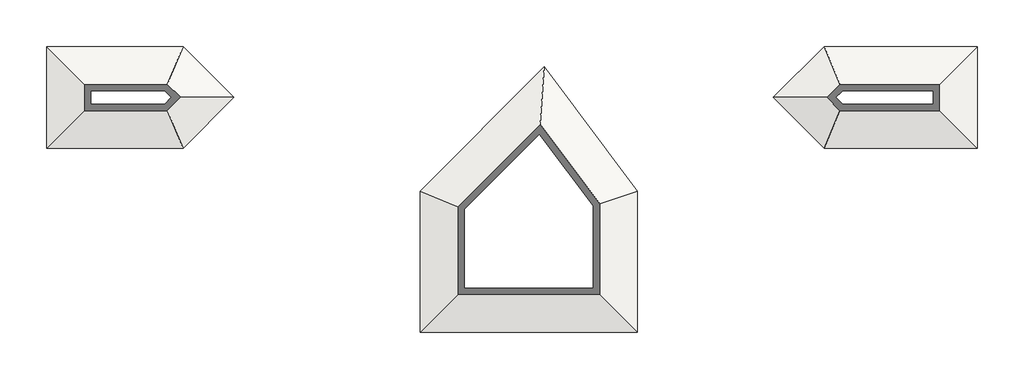
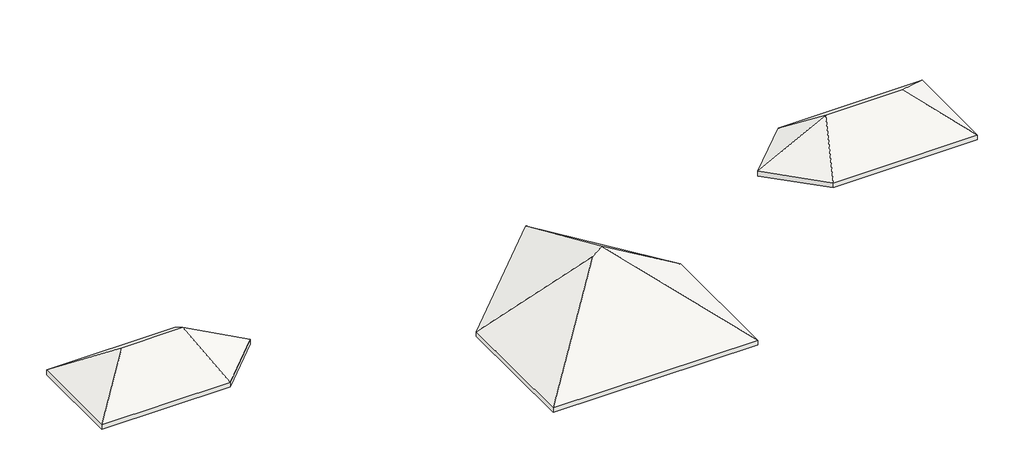
# One storey: 3 roofs.
"""IFC4 building model written with IfcOpenShell, lengths in millimetres."""

from ifc_helpers import new_model, si_unit, origin, place, context, project, spatial, faceted_brep, element, save

model = new_model("IFC4")

# Units and contexts
model_context = context("Model", 3, world=origin())
ifc_project = project(units=[si_unit("LENGTHUNIT", "METRE", prefix="MILLI")], contexts=[model_context])

# Site, building, storey
site = spatial("IfcSite", under=ifc_project)
building = spatial("IfcBuilding", under=site)
storey = spatial("IfcBuildingStorey", under=building, Elevation=7500.0)

# Roofs
placement = place(None, origin())
element("IfcRoof", 1, ObjectType="01-roof sheet", at=placement, inside=storey, context=model_context, shape_type="Brep", body=[
    faceted_brep([(-11618.9169632, -3415.5592374, 7500.0), (-6716.8860603, -3415.5592374, 7500.0), (-7472.8258116, -5240.5592374, 8868.75), (-9793.9169632, -5240.5592374, 8868.75), (-11618.9169632, -7065.5592374, 7500.0), (-6716.8860603, -7065.5592374, 7500.0), (-4891.8860603, -5240.5592374, 7500.0), (-11618.9169632, -3415.5592374, 7687.5), (-9793.9169632, -5240.5592374, 9056.25), (-7472.8258116, -5240.5592374, 9056.25), (-6716.8860603, -3415.5592374, 7687.5), (-11618.9169632, -7065.5592374, 7687.5), (-6716.8860603, -7065.5592374, 7687.5), (-4891.8860603, -5240.5592374, 7687.5)], [[[0, 1, 2, 3]], [[0, 3, 4]], [[4, 3, 2, 5]], [[6, 2, 1]], [[5, 2, 6]], [[7, 8, 9, 10]], [[7, 11, 8]], [[11, 12, 9, 8]], [[13, 10, 9]], [[12, 13, 9]], [[4, 11, 7, 0]], [[5, 12, 11, 4]], [[6, 13, 12, 5]], [[1, 10, 13, 6]], [[0, 7, 10, 1]]]),
])
element("IfcRoof", 2, ObjectType="01-roof sheet", at=placement, inside=storey, context=model_context, shape_type="Brep", body=[
    faceted_brep([(19981.0830368, -5240.5592374, 8868.75), (21806.0830368, -7065.5592374, 7500.0), (16306.0830368, -7065.5592374, 7500.0), (17062.0227881, -5240.5592374, 8868.75), (21806.0830368, -3415.5592374, 7500.0), (16306.0830368, -3415.5592374, 7500.0), (14481.0830368, -5240.5592374, 7500.0), (21806.0830368, -7065.5592374, 7687.5), (19981.0830368, -5240.5592374, 9056.25), (17062.0227881, -5240.5592374, 9056.25), (16306.0830368, -7065.5592374, 7687.5), (21806.0830368, -3415.5592374, 7687.5), (16306.0830368, -3415.5592374, 7687.5), (14481.0830368, -5240.5592374, 7687.5)], [[[0, 1, 2, 3]], [[4, 0, 3, 5]], [[1, 0, 4]], [[6, 3, 2]], [[5, 3, 6]], [[7, 8, 9, 10]], [[11, 12, 9, 8]], [[7, 11, 8]], [[13, 10, 9]], [[12, 13, 9]], [[4, 11, 7, 1]], [[5, 12, 11, 4]], [[6, 13, 12, 5]], [[2, 10, 13, 6]], [[1, 7, 10, 2]]]),
])
element("IfcRoof", 3, ObjectType="01-roof sheet", at=placement, inside=storey, context=model_context, shape_type="Brep", body=[
    faceted_brep([(9593.5830368, -8603.0592374, 7500.0), (9593.5830368, -13678.0592374, 7500.0), (5822.5828445, -9907.0590452, 10328.2501442), (5844.5730898, -9853.9698969, 10311.7574602), (1793.5830368, -8603.0592374, 7500.0), (5382.1499513, -10089.4923229, 10191.4251859), (1793.5830368, -13678.0592374, 7500.0), (6248.3557582, -4148.286516, 7500.0), (9593.5830368, -8603.0592374, 7687.5), (5844.5730898, -9853.9698969, 10499.2574602), (5822.5828445, -9907.0590452, 10515.7501442), (9593.5830368, -13678.0592374, 7687.5), (1793.5830368, -8603.0592374, 7687.5), (1793.5830368, -13678.0592374, 7687.5), (5382.1499513, -10089.4923229, 10378.9251859), (6248.3557582, -4148.286516, 7687.5)], [[[0, 1, 2, 3]], [[4, 5, 6]], [[7, 3, 2, 5, 4]], [[0, 3, 7]], [[6, 5, 2, 1]], [[8, 9, 10, 11]], [[12, 13, 14]], [[15, 12, 14, 10, 9]], [[8, 15, 9]], [[13, 11, 10, 14]], [[7, 15, 8, 0]], [[4, 12, 15, 7]], [[6, 13, 12, 4]], [[1, 11, 13, 6]], [[0, 8, 11, 1]]]),
])

save(model, "model.ifc")

# Revit data of these elements
# Type "01-roof sheet"
#   Description = "Generic Roof (Material By Category), 225mm thick"
#   Assembly Code = "B1020"
#   Type Mark = "G01"
#   Layers, outside or top first: 150 mm "roof" (function 1)
# Elements 1, 2 (IfcRoof, "01-roof sheet")
#   built-in parameter 1001705 = 29.7121 (stored number, unit not read)
#   built-in parameter 1001710 = 33615
#   Phase Created = New Construction
#   Materials on its faces: "roof"
# Element 3 (IfcRoof, "01-roof sheet")
#   built-in parameter 1001705 = 34.5005 (stored number, unit not read)
#   built-in parameter 1001710 = 33615
#   Phase Created = New Construction
#   Materials on its faces: "roof"
# Materials
#   "roof": class "Generic", colour RGB 120 120 120, transparency 0, Cost = 0
